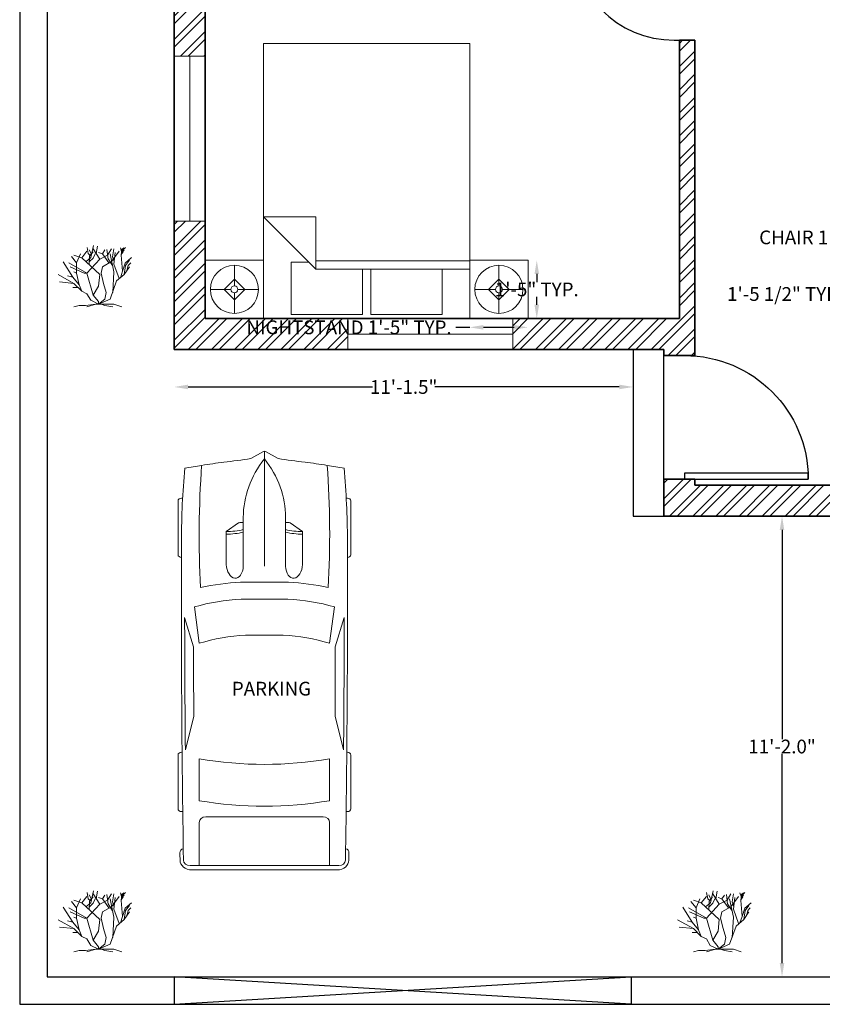
# Model space of a CAD drawing. Units: inches. Extents: x 0 to 478, y -33 to 633.
# Tile 1 of 4: x 0 to 234, y 0 to 286. Entities that reach past the tile are written whole.
import ezdxf

# ---------------------------------------------------------------- set-up
doc = ezdxf.new("R2010")
doc.units = ezdxf.units.IN
for name, color, linetype, lineweight in [('A-ANNO-DIMS', 2, 'Continuous', 18), ('A-AREA-IDEN', 7, 'Continuous', 18), ('A-DOOR', 3, 'Continuous', 25), ('A-FLOR-STRS', 7, 'Continuous', 25), ('A-FURN', 8, 'Continuous', 18), ('A-GLAZ', 4, 'Continuous', 18), ('A-WALL', 7, 'Continuous', 35), ('A-WALL-PATT', 252, 'Continuous', 13), ('C-PRKG', 8, 'Continuous', 18), ('C-PROP', 7, 'Continuous', 30), ('L-PLNT', 3, 'Continuous', 18)]:
    doc.layers.add(name, color=color, linetype=linetype, lineweight=lineweight)
doc.styles.get("Standard").update_dxf_attribs({"font": 'arial.ttf'})
doc.dimstyles.get("Standard").update_dxf_attribs({"dimtxt": 4, "dimasz": 4, "dimexe": 0.18, "dimexo": 0.0625, "dimgap": 0.09, "dimtad": 0, "dimtih": 1, "dimtoh": 1, "dimdec": 1, "dimzin": 0, "dimdsep": 46, "dimlunit": 3, "dimtxsty": 'Standard', "dimcen": 0.09, "dimse1": 1, "dimse2": 1, "dimadec": 0, "dimazin": 0, "dimtfac": 1, "dimtdec": 1, "dimtofl": 0, "dimtmove": 0, "dimatfit": 3, "dimfxl": 1, "dimtolj": 1, "dimtzin": 0, "dimarcsym": 0})

# ---------------------------------------------------------------- blocks, each defined once
blk = doc.blocks.new('Bed - Queen')
for p, q in [((0, -80.00003), (0, 0)), ((0, 0), (59.99999, 0)), ((59.99999, 0), (59.99999, -80.00003)), ((7.99999, -1.2), (28.79998, -1.2)), ((7.99999, -14.4), (7.99999, -1.2)), ((28.79998, -1.2), (28.79998, -14.4)), ((31.19999, -1.2), (51.99999, -1.2)), ((31.19999, -14.4), (31.19999, -1.2)), ((51.99999, -1.2), (51.99999, -16.4)), ((0, -14.4), (44.8, -14.4)), ((44.8, -16.8), (0, -16.8)), ((59.99999, -29.6), (44.8, -14.4)), ((44.8, -14.4), (44.8, -29.6)), ((51.99999, -16.4), (46.79936, -16.4)), ((44.8, -29.6), (59.99999, -29.6)), ((59.99999, -80.00003), (0, -80.00003))]:
    blk.add_line(p, q)
blk = doc.blocks.new('*U15')
for p, q in [((-30, 0), (-30, -6)), ((0, 0), (0, -6))]:
    blk.add_line(p, q)
blk.add_lwpolyline([(0, 0), (0, 30), (-1.75, 30), (-1.75, 0)], close=True)
blk.add_arc((0, 0), 30, 90, 180)
blk = doc.blocks.new('*U16')
for p, q in [((0, 0), (0, -6)), ((36, 0), (36, -6))]:
    blk.add_line(p, q)
blk.add_lwpolyline([(0, 0), (0, 36), (1.75, 36), (1.75, 0)], close=True)
blk.add_arc((0, 0), 36, 0, 90)
blk = doc.blocks.new('Shrub - elevation')
for p, q in [((-12.471, 19.775), (-12.898, 22.044)), ((-11.433, 18.289), (-10.457, 22.749)), ((-9.48, 19.775), (-8.992, 22.592)), ((0.041, 20.714), (1.384, 22.044)), ((-16.8, 16.32), (-18.72, 18.72)), ((-14.88, 18.24), (-17.76, 19.2)), ((-16.8, 16.32), (-15.36, 19.68)), ((-14.88, 18.24), (-12.96, 20.64)), ((-11.677, 19.071), (-12.471, 19.775)), ((-11.28, 19.619), (-12.104, 21.184)), ((-12.043, 15.628), (-11.921, 18.836)), ((-11.921, 18.836), (-10.64, 20.401)), ((-10.579, 18.054), (-9.846, 19.697)), ((-8.16, 17.76), (-10.56, 21.6)), ((-7.2, 19.68), (-8.64, 20.16)), ((-8.16, 17.76), (-5.28, 19.2)), ((-7.2, 19.68), (-6.24, 21.12)), ((-4.8, 16.32), (-7.2, 19.68)), ((-5.086, 17.741), (-5.513, 21.34)), ((-5.28, 19.2), (-3.84, 21.6)), ((-2.88, 12.96), (-4.32, 19.68)), ((-3.84, 16.8), (-0.96, 20.64)), ((-3.377, 18.602), (-2.888, 21.575)), ((-2.766, 16.802), (-3.377, 18.602)), ((-2.88, 15.84), (-2.4, 20.16)), ((-0.508, 21.888), (-0.081, 20.558)), ((-0.203, 19.149), (0.102, 21.34)), ((0.346, 13.203), (-0.203, 19.149)), ((-0.142, 19.384), (0.59, 20.401)), ((-0.02, 20.01), (0.896, 21.105)), ((0.102, 21.34), (0.835, 21.888)), ((-18.24, 11.04), (-21.755, 16.655)), ((-12.96, 12.48), (-19.68, 16.32)), ((-13.92, 12.48), (-19.2, 14.88)), ((-16.8, 12.48), (-16.8, 16.32)), ((-8.16, 12), (-14.88, 18.24)), ((-13.325, 16.724), (-11.433, 18.289)), ((-12.96, 12.48), (-8.16, 17.76)), ((-11.982, 16.802), (-10.579, 18.054)), ((-7.68, 12.48), (-7.2, 14.88)), ((-7.2, 14.88), (-3.84, 16.8)), ((-3.377, 15.315), (-5.086, 17.819)), ((-0.96, 10.56), (-2.88, 15.84)), ((0.346, 13.203), (1.323, 16.254)), ((0.96, 12), (1.44, 15.36)), ((0.96, 12), (2.88, 14.88)), ((1.323, 16.254), (3.642, 18.289)), ((1.44, 15.36), (2.88, 17.28)), ((1.92, 13.44), (2.4, 15.36)), ((2.4, 15.36), (3.36, 16.32)), ((-17.76, 8.64), (-23.663, 11.961)), ((-18.24, 11.04), (-20.16, 11.52)), ((-15.84, 8.16), (-18.24, 11.04)), ((-16.8, 12.48), (-17.76, 12.96)), ((-15.84, 8.16), (-16.8, 12.48)), ((-12.96, 12.48), (-13.92, 12.48)), ((-10.56, 4.32), (-12.96, 12.48)), ((-8.64, 7.68), (-8.16, 12)), ((-6.72, 8.64), (-7.68, 12.48)), ((-3.36, 5.28), (-2.88, 12.96)), ((-1.92, 9.6), (0.96, 12)), ((-0.48, 10.8), (0.346, 13.203)), ((-17.76, 8.64), (-23.128, 9.222)), ((-14.88, 5.76), (-17.76, 8.64)), ((-14.88, 5.76), (-15.84, 8.16)), ((-10.56, 4.32), (-8.64, 7.68)), ((-5.76, 5.28), (-6.72, 8.64)), ((-4.32, 2.88), (-1.92, 9.6)), ((-16.32, 7.2), (-18.24, 7.2)), ((-12.96, 4.8), (-14.88, 5.76)), ((-11.52, 2.4), (-12.96, 4.8)), ((-8.64, 1.92), (-10.56, 4.32)), ((-6.24, 2.88), (-5.76, 5.28)), ((-15.84, 0.48), (-17.76, 0)), ((-13.44, 0.48), (-15.84, 0.48)), ((-9.6, 0.96), (-13.44, 0.48)), ((-9.6, 0.96), (-12.96, 0)), ((-8.64, 0.96), (-11.52, 2.4)), ((-9.6, 0.96), (-7.68, 0.96)), ((-8.64, 0.96), (-4.32, 2.88)), ((-8.64, 0.96), (-6.24, 2.88)), ((-8.64, 0.96), (-8.64, 1.92)), ((-8.64, 0.96), (-2.88, 0.96)), ((-7.68, 0.96), (-6.24, 0.48)), ((-6.24, 0.48), (-3.36, 0)), ((-2.88, 0.96), (0, 0))]:
    blk.add_line(p, q)
blk = doc.blocks.new('*U18')
for p, q in [((21.1, 37.41), (21.1, 36.83)), ((46.55, 38.89), (22.35, 38.89)), ((47.8, 37.39), (47.8, 37.41)), ((87.99, 31.87), (74.76, 35.92)), ((134.31, 35.6), (119.29, 31.78)), ((135.45, 37.07), (135.45, 37.41)), ((136.7, 38.89), (160.9, 38.89)), ((162.15, 37.41), (162.15, 36.77)), ((70.03, 31.54), (86.41, 29.35)), ((186.47, -33.5), (186.47, 33.5)), ((188.4, -32.76), (188.4, 32.76)), ((138.42, 29.35), (157.25, 29.35)), ((186.47, 29.35), (167.01, 29.35)), ((164.52, 26.39), (164.52, -26.39)), ((32.27, 11.63), (36.13, 17.17)), ((36.13, 17.17), (50.94, 17.17)), ((29.77, 9.51), (51.68, 9.51)), ((32.12, 9.51), (32.12, 11.15)), ((58.92, -10.77), (58.92, 10.77)), ((66.55, -10.53), (66.55, 10.53)), ((186.47, -10.53), (186.47, 10.53)), ((3.27, 6.13), (0.1, 0.41)), ((82.74, 8.5), (82.74, -8.5)), ((0, 0), (51.68, 0)), ((0.1, -0.41), (3.27, -6.13)), ((29.77, -9.51), (51.68, -9.51)), ((32.12, -9.51), (32.12, -11.15)), ((32.27, -11.63), (36.13, -17.17)), ((36.13, -17.17), (50.94, -17.17)), ((86.41, -29.35), (70.03, -31.54)), ((157.25, -29.35), (138.42, -29.35)), ((167.01, -29.35), (186.47, -29.35)), ((87.99, -31.87), (74.76, -35.92)), ((134.31, -35.6), (119.29, -31.78)), ((21.1, -37.41), (21.1, -36.83)), ((46.55, -38.89), (22.35, -38.89)), ((47.8, -37.39), (47.8, -37.41)), ((135.45, -37.07), (135.45, -37.41)), ((136.7, -38.89), (160.9, -38.89)), ((162.15, -37.41), (162.15, -36.77))]:
    blk.add_line(p, q)
for centre, major_axis, ratio, start_param, end_param in [((266.03, -27.52), (0, 313.31), 0.842304, 1.367076, 1.39176), ((41.19, -490.86), (0, 528.23), 0.842304, 0.00281, 0.075598), ((22.35, 37.41), (0, -1.48), 0.842304, 3.141593, 4.712389), ((64.48, -10555.62), (0, 10593.03), 0.842304, -0.013397, 0.002797), ((46.55, 37.41), (0, 1.48), 0.842304, -1.570796, 0), ((64.48, -10555.62), (0, -10591.55), 0.842304, 3.133765, 3.140441), ((136.7, 37.41), (0, -1.48), 0.842304, 3.141593, 4.712389), ((160.9, 37.41), (0, 1.48), 0.842304, -1.570796, 0), ((180.63, 35.84), (0, 2.22), 0.842304, -0.013017, 1.249894), ((64.48, -10556.36), (0, 10595.31), 0.842304, -0.013397, -0.013017), ((183.98, 33.5), (0, -2.96), 0.842304, 1.570796, 3.128196), ((183.98, 32.76), (0, -5.25), 0.842304, 1.570796, 3.128196), ((135.29, 5.39), (0, 81.77), 0.842304, 1.245306, 1.50788), ((95.79, -3666.35), (0, -3698.24), 0.842304, 3.134049, 3.144098), ((259.18, -27.52), (0, -305.3), 0.842304, 4.528606, 4.561838), ((37.47, -593.96), (0, -623.33), 0.842304, 3.096046, 3.200911), ((134.4, 5.39), (0, -89.78), 0.842304, 4.449482, 4.652344), ((149.6, 2.8), (0, -79.58), 0.842304, 4.372215, 4.640744), ((17.08, 0), (0, 147.02), 0.842304, 4.511394, 4.913384), ((35.91, 0), (0, 147.02), 0.842304, 4.511394, 4.913384), ((167.01, 26.39), (0, 2.96), 0.842304, 0, 1.570796), ((-204.49, 52.4), (0, -250.96), 0.842304, 1.385369, 1.434372), ((13.04, 17.01), (0, 27.42), 0.842304, 4.435146, 4.718221), ((14.2, 17.01), (0, 27.42), 0.842304, 4.435146, 4.718221), ((50.79, 13.34), (6.34, -0.36), 0.603834, -1.395552, 1.581315), ((29.77, -46.66), (0, 56.17), 0.842304, 0, 0.590319), ((32.75, 11.15), (0, 0.74), 0.842304, 0.879714, 1.570796), ((0.62, 0), (0, -0.74), 0.842304, 4.131459, 5.293319), ((29.77, 46.66), (0, 56.17), 0.842304, 2.551274, 3.141593), ((-204.49, -52.4), (0, 250.96), 0.842304, -1.434372, -1.385369), ((149.6, -2.8), (0, -79.58), 0.842304, -1.499151, -1.230623), ((32.75, -11.15), (0, -0.74), 0.842304, 4.712389, 5.403472), ((13.04, -17.01), (0, -27.42), 0.842304, 1.564964, 1.848039), ((14.2, -17.01), (0, -27.42), 0.842304, 1.564964, 1.848039), ((134.4, -5.39), (0, -89.78), 0.842304, -1.510751, -1.307889), ((135.29, -5.39), (0, -81.77), 0.842304, -1.50788, -1.245306), ((259.18, 27.52), (0, 305.3), 0.842304, 1.721348, 1.754579), ((167.01, -26.39), (0, -2.96), 0.842304, 4.712389, 6.283185), ((266.03, 27.52), (0, 313.31), 0.842304, 1.749832, 1.774517), ((37.47, 593.96), (0, -623.33), 0.842304, -0.059319, 0.045547), ((95.79, 3666.35), (0, -3698.24), 0.842304, -0.002505, 0.007544), ((183.98, -33.5), (0, 2.96), 0.842304, 3.15499, 4.712389), ((183.98, -32.76), (0, -5.25), 0.842304, 0.013397, 1.570796), ((41.19, 490.86), (0, -528.23), 0.842304, -0.075598, -0.00281), ((22.35, -37.41), (0, 1.48), 0.842304, 1.570796, 3.141593), ((64.48, 10555.62), (0, 10593.03), 0.842304, 3.138796, 3.15499), ((46.55, -37.41), (0, -1.48), 0.842304, 0, 1.570796), ((64.48, 10555.62), (0, -10591.55), 0.842304, 0.001152, 0.007828), ((136.7, -37.41), (0, -1.48), 0.842304, -1.570796, 0), ((160.9, -37.41), (0, 1.48), 0.842304, 3.141593, 4.712389), ((180.63, -35.84), (0, -2.22), 0.842304, -1.249894, 0.013017), ((64.48, 10556.36), (0, 10595.31), 0.842304, 3.15461, 3.15499)]:
    blk.add_ellipse(centre, major_axis=major_axis, ratio=ratio, start_param=start_param, end_param=end_param)
at = {"extrusion": (0, 0, -1)}
blk.add_ellipse((50.79, -13.34), major_axis=(6.34, 0.36), ratio=0.603834, start_param=-1.395552, end_param=1.581315, dxfattribs=at)
blk = doc.blocks.new('*D19')
at = {"layer": 'A-ANNO-DIMS', "color": 0, "lineweight": -2, "transparency": 16777216}
for p, q in [((221.86, 138), (221.86, 77.13)), ((221.86, 12), (221.86, 72.87))]:
    blk.add_line(p, q, dxfattribs=at)
at = {"layer": 'A-ANNO-DIMS', "color": 0, "transparency": 16777216}
for points in [[(221.19, 138), (222.52, 138), (221.86, 142)], [(221.19, 12), (222.52, 12), (221.86, 8)]]:
    blk.add_solid(points, dxfattribs=at)
at = {"layer": 'Defpoints', "color": 0, "transparency": 16777216}
for p in [(187.5, 142), (187.5, 8), (221.86, 8)]:
    blk.add_point(p, dxfattribs=at)
at = {"layer": 'A-ANNO-DIMS', "color": 0, "transparency": 16777216, "insert": (221.86, 75), "char_height": 4, "attachment_point": 5}
blk.add_mtext('\\A1;11\'-2.0"', dxfattribs=at)
blk = doc.blocks.new('*D21')
at = {"layer": 'A-ANNO-DIMS', "color": 0, "lineweight": -2, "transparency": 16777216}
for p, q in [((49, 179.6), (102.65, 179.6)), ((174.5, 179.6), (120.85, 179.6))]:
    blk.add_line(p, q, dxfattribs=at)
at = {"layer": 'A-ANNO-DIMS', "color": 0, "transparency": 16777216}
for points in [[(49, 180.27), (49, 178.94), (45, 179.6)], [(174.5, 180.27), (174.5, 178.94), (178.5, 179.6)]]:
    blk.add_solid(points, dxfattribs=at)
at = {"layer": 'Defpoints', "color": 0, "transparency": 16777216}
for p in [(45, 190.5), (178.5, 190.5), (178.5, 179.6)]:
    blk.add_point(p, dxfattribs=at)
at = {"layer": 'A-ANNO-DIMS', "color": 0, "transparency": 16777216, "insert": (111.75, 179.6), "char_height": 4, "attachment_point": 5}
blk.add_mtext('\\A1;11\'-1.5"', dxfattribs=at)
blk = doc.blocks.new('WIN-48IN')
for p, q in [((0, 48), (9, 48)), ((4.5, 48), (4.5, 0)), ((0, 0), (9, 0))]:
    blk.add_line(p, q)
blk = doc.blocks.new('Lamp - Table')
for p, q in [((0, 7), (0, 1)), ((0, 3), (-3, 0)), ((3, 0), (0, 3)), ((-1, 0), (-7, 0)), ((-3, 0), (0, -3)), ((0, -3), (3, 0)), ((1, 0), (7, 0)), ((0, -1), (0, -7))]:
    blk.add_line(p, q)
for radius in [7, 1]:
    blk.add_circle((0, 0), radius)
blk = doc.blocks.new('END-TABLE-WITH-LAMP')
blk.add_lwpolyline([(-8.49, 8.49), (-8.49, -8.49), (8.49, -8.49), (8.49, 8.49)], close=True)
blk.add_blockref('Lamp - Table', (0, 0))
blk = doc.blocks.new('*D32')
at = {"layer": 'A-ANNO-DIMS', "color": 0, "lineweight": -2, "transparency": 16777216}
for p, q in [((130.97, 196.95), (126.97, 196.95)), ((143.94, 196.95), (134.97, 196.95))]:
    blk.add_line(p, q, dxfattribs=at)
at = {"layer": 'A-ANNO-DIMS', "color": 0, "transparency": 16777216}
for points in [[(134.97, 197.62), (134.97, 196.29), (130.97, 196.95)], [(143.94, 197.62), (143.94, 196.29), (147.94, 196.95)]]:
    blk.add_solid(points, dxfattribs=at)
at = {"layer": 'Defpoints', "color": 0, "transparency": 16777216}
for p in [(130.97, 199.5), (147.94, 199.5), (130.97, 196.95)]:
    blk.add_point(p, dxfattribs=at)
at = {"layer": 'A-ANNO-DIMS', "color": 0, "transparency": 16777216, "insert": (95.85, 196.95), "char_height": 4, "attachment_point": 5}
blk.add_mtext('\\A1;NIGHTSTAND 1\'-5" TYP.', dxfattribs=at)
blk = doc.blocks.new('*D33')
at = {"layer": 'A-ANNO-DIMS', "color": 0, "lineweight": -2, "transparency": 16777216}
for p, q in [((150.49, 212.47), (150.49, 210.12)), ((150.49, 203.5), (150.49, 205.85))]:
    blk.add_line(p, q, dxfattribs=at)
at = {"layer": 'A-ANNO-DIMS', "color": 0, "transparency": 16777216}
for points in [[(149.82, 212.47), (151.15, 212.47), (150.49, 216.47)], [(149.82, 203.5), (151.15, 203.5), (150.49, 199.5)]]:
    blk.add_solid(points, dxfattribs=at)
at = {"layer": 'Defpoints', "color": 0, "transparency": 16777216}
for p in [(147.94, 216.47), (147.94, 199.5), (150.49, 199.5)]:
    blk.add_point(p, dxfattribs=at)
at = {"layer": 'A-ANNO-DIMS', "color": 0, "transparency": 16777216, "insert": (150.49, 207.99), "char_height": 4, "attachment_point": 5}
blk.add_mtext('\\A1;1\'-5" TYP.', dxfattribs=at)
blk = doc.blocks.new('*D44')
at = {"layer": 'A-ANNO-DIMS', "color": 0, "lineweight": -2, "transparency": 16777216}
for p, q in [((261.68, 223.12), (257.68, 223.12)), ((264.27, 220.07), (261.68, 223.12)), ((275.25, 207.09), (266.85, 217.01))]:
    blk.add_line(p, q, dxfattribs=at)
at = {"layer": 'A-ANNO-DIMS', "color": 0, "transparency": 16777216}
for points in [[(267.36, 217.44), (266.34, 216.58), (264.27, 220.07)], [(275.76, 207.53), (274.74, 206.66), (277.84, 204.04)]]:
    blk.add_solid(points, dxfattribs=at)
at = {"layer": 'Defpoints', "color": 0, "transparency": 16777216}
for p in [(261.86, 218.03), (264.27, 220.07), (275.43, 202.01)]:
    blk.add_point(p, dxfattribs=at)
at = {"layer": 'A-ANNO-DIMS', "color": 0, "transparency": 16777216, "insert": (235.95, 223.12), "char_height": 4, "attachment_point": 5}
blk.add_mtext('\\A1;CHAIR 1\'-9" TYP.', dxfattribs=at)
blk = doc.blocks.new('*D45')
at = {"layer": 'A-ANNO-DIMS', "color": 0, "lineweight": -2, "transparency": 16777216}
for p, q in [((256.77, 217.85), (249.65, 211.82)), ((246.6, 209.23), (243.55, 206.65)), ((243.55, 206.65), (239.55, 206.65))]:
    blk.add_line(p, q, dxfattribs=at)
at = {"layer": 'A-ANNO-DIMS', "color": 0, "transparency": 16777216}
for points in [[(256.34, 218.36), (257.2, 217.34), (259.83, 220.43)], [(249.22, 212.32), (250.08, 211.31), (246.6, 209.23)]]:
    blk.add_solid(points, dxfattribs=at)
at = {"layer": 'Defpoints', "color": 0, "transparency": 16777216}
for p in [(261.86, 218.03), (246.6, 209.23), (248.64, 206.83)]:
    blk.add_point(p, dxfattribs=at)
at = {"layer": 'A-ANNO-DIMS', "color": 0, "transparency": 16777216, "insert": (222.79, 206.65), "char_height": 4, "attachment_point": 5}
blk.add_mtext('\\A1;1\'-5 1/2" TYP.', dxfattribs=at)
blk = doc.blocks.new('*D55')
at = {"layer": 'A-ANNO-DIMS', "color": 0, "lineweight": -2, "transparency": 16777216}
for p, q in [((197.5, 630.8), (206.09, 630.8)), ((225.5, 630.8), (216.91, 630.8))]:
    blk.add_line(p, q, dxfattribs=at)
at = {"layer": 'A-ANNO-DIMS', "color": 0, "transparency": 16777216}
for points in [[(197.5, 631.47), (197.5, 630.13), (193.5, 630.8)], [(225.5, 631.47), (225.5, 630.13), (229.5, 630.8)]]:
    blk.add_solid(points, dxfattribs=at)
at = {"layer": 'Defpoints', "color": 0, "transparency": 16777216}
for p in [(229.5, 630.8), (193.5, 154.5), (229.5, 154.5)]:
    blk.add_point(p, dxfattribs=at)
at = {"layer": 'A-ANNO-DIMS', "color": 0, "transparency": 16777216, "insert": (211.5, 630.8), "char_height": 4, "attachment_point": 5}
blk.add_mtext('\\A1;3\'-0"', dxfattribs=at)

msp = doc.modelspace()

# ---------------------------------------------------------------- hatches: boundary and pattern name
at = {"layer": 'A-WALL-PATT'}
h = msp.add_hatch(dxfattribs=at)
h.set_pattern_fill('ANSI32', color=256, scale=0.5)
h.paths.add_polyline_path([(456, 600), (45, 600), (45, 547.04), (54, 547.04), (54, 591), (447, 591), (447, 507), (433.5, 507), (433.5, 498), (456, 498)])
h.paths.add_polyline_path([(54, 499.04), (45, 499.04), (45, 429), (54, 429)])
h.paths.add_polyline_path([(235.5, 453), (226.5, 453), (226.5, 591), (222, 591), (222, 453), (213, 453), (213, 448.5), (235.5, 448.5)])
h.paths.add_polyline_path([(105, 453), (54, 453), (54, 448.5), (105, 448.5)], flags=17)
h.paths.add_polyline_path([(183, 453), (129, 453), (129, 448.5), (138, 448.5), (138, 388.5), (54, 388.5), (54, 384), (138, 384), (138, 324), (129, 324), (129, 319.5), (192, 319.5), (192, 310.5), (196.5, 310.5), (196.5, 324), (142.5, 324), (142.5, 448.5), (183, 448.5)])
h.paths.add_polyline_path([(403.5, 453), (265.5, 453), (265.5, 448.5), (394.5, 448.5), (394.5, 442.5), (397.5, 442.5), (403.5, 442.5)])
h.paths.add_polyline_path([(412.5, 507), (399, 507), (399, 558), (394.5, 558), (394.5, 498), (412.5, 498)], flags=17)
h.paths.add_polyline_path([(399, 591), (394.5, 591), (394.5, 582), (399, 582)], flags=17)
h.paths.add_polyline_path([(54, 408), (45, 408), (45, 364.5), (54, 364.5)])
h.paths.add_polyline_path([(54, 343.5), (45, 343.5), (45, 275.82), (54, 275.82), (54, 319.5)])
h.paths.add_polyline_path([(105, 324), (54, 324), (54, 319.5), (105, 319.5)], flags=17)
h.paths.add_polyline_path([(403.5, 412.5), (397.5, 412.5), (394.5, 412.5), (394.5, 388.53), (403.5, 388.53)])
h.paths.add_polyline_path([(403.5, 340.53), (394.5, 340.53), (394.5, 311.5), (256.5, 311.5), (256.5, 307), (394.5, 307), (394.5, 255.85), (403.5, 255.85)])
h.paths.add_polyline_path([(54, 216.47), (54, 227.82), (45, 227.82), (45, 190.5), (95.47, 190.5), (95.47, 199.5), (70.97, 199.5), (54, 199.5)])
h.paths.add_polyline_path([(196.5, 280.5), (192, 280.5), (192, 199.5), (143.47, 199.5), (143.47, 190.5), (187.5, 190.5), (187.5, 188.75), (193.5, 188.75), (196.5, 188.75)])
h.paths.add_polyline_path([(403.5, 207.85), (394.5, 207.85), (394.5, 126.5), (403.5, 126.5)])
h.paths.add_polyline_path([(403.5, 78.5), (394.5, 78.5), (394.5, 63), (265.7, 63), (265.7, 54), (403.5, 54)])
h.paths.add_polyline_path([(394.5, 151), (313.7, 151), (313.7, 142), (394.5, 142)])
h.paths.add_polyline_path([(265.7, 151), (196.5, 151), (196.5, 152.75), (193.5, 152.75), (187.5, 152.75), (187.5, 142), (265.7, 142)])

# ---------------------------------------------------------------- linework, layer by layer
at = {"layer": 'A-FLOR-STRS'}
msp.add_lwpolyline([(187.5, 190.5), (178.5, 190.5), (178.5, 142), (187.5, 142)], close=True, dxfattribs=at)
at = {"layer": 'A-WALL'}
for p, q in [((45, 600), (45, 190.5)), ((54, 591), (54, 199.5)), ((54, 319.5), (54, 199.5)), ((192, 280.5), (192, 199.5)), ((192, 280.5), (196.5, 280.5)), ((196.5, 280.5), (196.5, 188.75)), ((192, 199.5), (54, 199.5)), ((187.5, 190.5), (45, 190.5)), ((187.5, 190.5), (187.5, 188.75)), ((187.5, 188.75), (196.5, 188.75)), ((187.5, 152.75), (187.5, 142)), ((187.5, 152.75), (196.5, 152.75)), ((196.5, 152.75), (196.5, 151)), ((394.5, 151), (196.5, 151)), ((394.5, 142), (187.5, 142))]:
    msp.add_line(p, q, dxfattribs=at)
at = {"layer": 'C-PROP'}
for p, q in [((0, 600), (0, 0)), ((8, 592), (8, 8)), ((8, 8), (451.5, 8)), ((0, 0), (456, 0))]:
    msp.add_line(p, q, dxfattribs=at)
msp.add_lwpolyline([(45, 0), (178, 8), (178, 0), (45, 8)], close=True, dxfattribs=at)

# ---------------------------------------------------------------- block references
at = {"layer": 'A-DOOR', "rotation": 90.00000000000003}
msp.add_blockref('*U15', (190.5, 310.5), dxfattribs=at)
at = {"layer": 'A-DOOR', "xscale": -1, "rotation": 270}
msp.add_blockref('*U16', (193.5, 152.75), dxfattribs=at)
at = {"layer": 'A-FURN', "rotation": 180}
for name, p in [('Bed - Queen', (130.97, 199.5)), ('END-TABLE-WITH-LAMP', (139.46, 207.99))]:
    msp.add_blockref(name, p, dxfattribs=at)
at = {"layer": 'A-FURN', "extrusion": (0, 0, -1), "zscale": -1, "rotation": 180}
msp.add_blockref('END-TABLE-WITH-LAMP', (-62.49, 207.99), dxfattribs=at)
at = {"layer": 'A-GLAZ'}
msp.add_blockref('WIN-48IN', (45, 227.82), dxfattribs=at)
at = {"layer": 'A-GLAZ', "rotation": 269.9999999999999}
msp.add_blockref('WIN-48IN', (95.47, 199.5), dxfattribs=at)
at = {"layer": 'C-PRKG', "xscale": 0.6464620946967194, "yscale": 0.6464620946967194, "zscale": 0.6464620946967194, "rotation": 270}
msp.add_blockref('*U18', (71.23, 160.9), dxfattribs=at)
at = {"layer": 'L-PLNT', "xscale": 0.78234725202095, "yscale": 0.78234725202095, "zscale": 0.78234725202095}
for p in [(29.69, 202.93), (29.69, 15.26), (209.99, 15.26)]:
    msp.add_blockref('Shrub - elevation', p, dxfattribs=at)

# ---------------------------------------------------------------- texts
at = {"layer": 'A-AREA-IDEN', "ltscale": 0.5, "insert": (48.07, 93.83), "char_height": 4, "attachment_point": 1}
msp.add_mtext_dynamic_manual_height_columns('\\pxqc;PARKING', width=50.4232, gutter_width=12.5, heights=[0], dxfattribs=at)

# ---------------------------------------------------------------- dimensions: what is measured, and where the dimension line sits
at = {"layer": 'A-ANNO-DIMS'}
for base, p1, p2, override, picture, middle in [((229.5, 630.8), (193.5, 154.5), (229.5, 154.5), {"dimdec": 1, "dimlfac": 1, "dimrnd": 0, "dimzin": 1, "dimdsep": 46, "dimlunit": 4, "dimfrac": 2}, '*D55', (211.5, 630.8)), ((178.5, 179.6), (45, 190.5), (178.5, 190.5), {"dimclrd": 0, "dimclre": 0, "dimclrt": 0}, '*D21', (111.75, 179.6))]:
    dim = msp.add_linear_dim(base=base, p1=p1, p2=p2, dimstyle='Standard', override=override, dxfattribs=at)
    dim.commit()
    dim.dimension.update_dxf_attribs({"geometry": picture, "text_midpoint": middle})
for base, p1, p2, angle, text, picture, middle in [((264.27, 220.07), (275.43, 202.01), (261.86, 218.03), 130.2662, 'CHAIR <> TYP.', '*D44', (235.95, 223.12)), ((246.6, 209.23), (261.86, 218.03), (248.64, 206.83), 220.2662, '<> TYP.', '*D45', (222.79, 206.65)), ((150.49, 199.5), (147.94, 216.47), (147.94, 199.5), 270, '<> TYP.', '*D33', (150.49, 207.99)), ((130.97, 196.95), (147.94, 199.5), (130.97, 199.5), 180, 'NIGHTSTAND <> TYP.', '*D32', (95.85, 196.95))]:
    dim = msp.add_linear_dim(base=base, p1=p1, p2=p2, angle=angle, text=text, dimstyle='Standard', override={"dimdec": 1, "dimlfac": 1, "dimrnd": 0, "dimzin": 1, "dimdsep": 46, "dimlunit": 4, "dimfrac": 2}, dxfattribs=at)
    dim.commit()
    dim.dimension.update_dxf_attribs({"geometry": picture, "text_midpoint": middle})
dim = msp.add_linear_dim(base=(221.86, 8), p1=(187.5, 142), p2=(187.5, 8), angle=90, dimstyle='Standard', override={"dimclrd": 0, "dimclre": 0, "dimclrt": 0}, dxfattribs=at)
dim.commit()
dim.dimension.update_dxf_attribs({"geometry": '*D19', "text_midpoint": (221.86, 75)})

doc.saveas('drawing.dxf')
